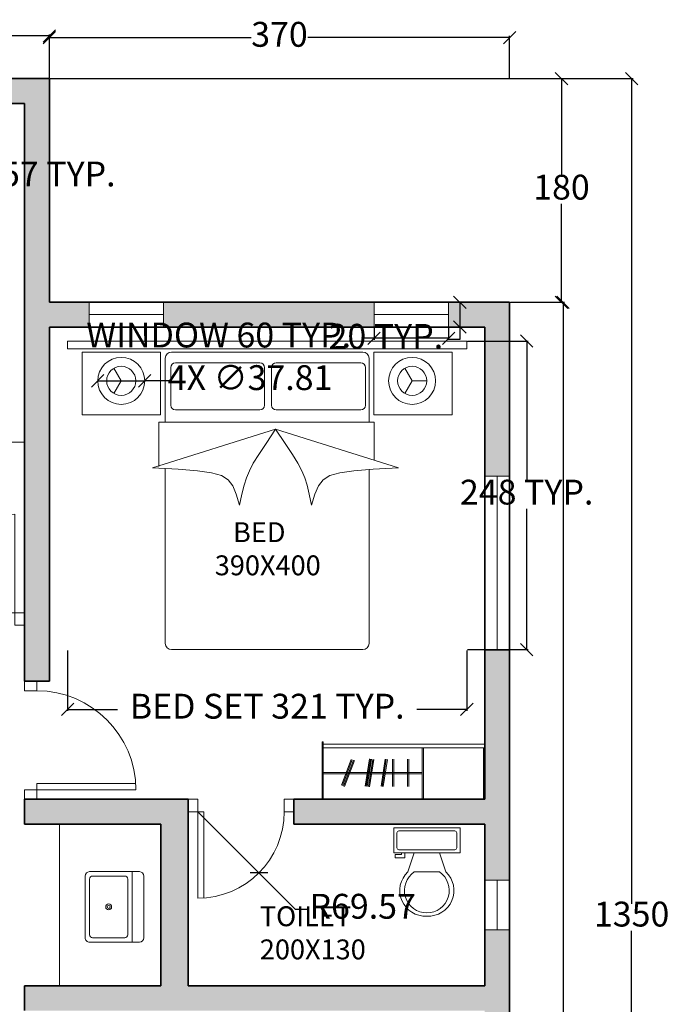
# Model space of a CAD drawing. Units: centimetres. Extents: x 2069 to 3209, y 376 to 1989.
# Tile 3 of 3: x 2687 to 3209, y 1196 to 1989. Entities that reach past the tile are written whole.
import ezdxf

# ---------------------------------------------------------------- set-up
doc = ezdxf.new("R2010")
doc.units = ezdxf.units.CM
for name, color, linetype, lineweight in [('A-ANNO-DIMS', 2, 'Continuous', 18), ('A-AREA-IDEN', 7, 'Continuous', 25), ('A-DOOR', 3, 'Continuous', 18), ('A-FLOR-CASE', 8, 'Continuous', 18), ('A-FLOR-FIXT', 8, 'Continuous', 18), ('A-FURN', 8, 'Continuous', 18), ('A-GLAZ', 4, 'Continuous', 18), ('A-WALL', 7, 'Continuous', 35), ('A-WALL-PATT', 252, 'Continuous', 13)]:
    doc.layers.add(name, color=color, linetype=linetype, lineweight=lineweight)
doc.styles.add('ATTR', font='romans.shx', dxfattribs={"width": 0.8, "height": 1.075})
doc.styles.get("Standard").update_dxf_attribs({"font": 'arial.ttf'})
doc.dimstyles.new('ISO-25', dxfattribs={"dimtxt": 20, "dimasz": 10, "dimexe": 1.25, "dimexo": 0.625, "dimtad": 0, "dimtih": 1, "dimtoh": 1, "dimtxsty": 'Standard', "dimblk": 'OBLIQUE', "dimcen": 6, "dimadec": 0, "dimazin": 0, "dimtfac": 1, "dimtmove": 0, "dimatfit": 3, "dimldrblk": 'OBLIQUE', "dimfxl": 1, "dimarcsym": 0})

# ---------------------------------------------------------------- blocks, each defined once
blk = doc.blocks.new('CAMMAT')
for p, q in [((1.2731, 0), (-1.2731, 0)), ((1.2731, 0), (1.2731, -0.05)), ((-1.2731, 0), (-1.2731, -0.05)), ((1.2731, -0.05), (-1.2731, -0.05)), ((-1.18, -0.07), (-1.18, -0.47)), ((-1.18, -0.07), (-0.68, -0.07)), ((-0.68, -0.07), (-0.68, -0.47)), ((-0.65, -0.11), (-0.65, -0.5169)), ((0.61, -0.07), (-0.61, -0.07)), ((0.65, -0.11), (0.65, -0.5169)), ((0.68, -0.07), (0.68, -0.47)), ((0.68, -0.07), (1.18, -0.07)), ((1.18, -0.07), (1.18, -0.47)), ((-0.931, -0.2541), (-0.9775, -0.1737)), ((-0.6152, -0.1695), (-0.6152, -0.4095)), ((-0.0465, -0.1395), (-0.5852, -0.1395)), ((-0.0165, -0.1695), (-0.0165, -0.4095)), ((0.0274, -0.1695), (0.0274, -0.4095)), ((0.5962, -0.1395), (0.0574, -0.1395)), ((0.6262, -0.1695), (0.6262, -0.4095)), ((0.9242, -0.2541), (0.8777, -0.1737)), ((-0.931, -0.2541), (-0.9775, -0.3346)), ((-0.931, -0.2541), (-0.8381, -0.2541)), ((0.9242, -0.2541), (0.8777, -0.3346)), ((0.9242, -0.2541), (1.0171, -0.2541)), ((-0.0465, -0.4395), (-0.5852, -0.4395)), ((0.5962, -0.4395), (0.0574, -0.4395)), ((-1.18, -0.47), (-0.68, -0.47)), ((0.68, -0.47), (1.18, -0.47)), ((0.0535, -0.5623), (-0.7312, -0.8093)), ((-0.6904, -0.5169), (-0.6904, -0.8)), ((-0.6904, -0.5169), (0.6826, -0.5169)), ((0.0535, -0.5623), (0.8382, -0.8093)), ((0.6826, -0.5169), (0.6826, -0.7603)), ((-0.65, -0.8139), (-0.65, -1.93)), ((0.65, -0.8204), (0.65, -1.93)), ((0.61, -1.97), (-0.61, -1.97))]:
    blk.add_line(p, q)
for points in [[(-0.1761, -1.0476), (-0.161, -0.9772), (-0.1474, -0.921), (-0.1326, -0.8732), (-0.1139, -0.8282), (-0.0886, -0.7803), (-0.0541, -0.7238), (-0.0076, -0.653), (0.0535, -0.5623)], [(0.2832, -1.0476), (0.2681, -0.9772), (0.2545, -0.921), (0.2396, -0.8732), (0.2209, -0.8282), (0.1957, -0.7803), (0.1611, -0.7238), (0.1147, -0.653), (0.0535, -0.5623)], [(-0.7312, -0.8093), (-0.5683, -0.8185), (-0.4451, -0.828), (-0.3552, -0.8406), (-0.2919, -0.8591), (-0.2489, -0.8862), (-0.2196, -0.9248), (-0.1975, -0.9777), (-0.1761, -1.0476)], [(0.8382, -0.8093), (0.6753, -0.8185), (0.5522, -0.828), (0.4622, -0.8406), (0.399, -0.8591), (0.356, -0.8862), (0.3267, -0.9248), (0.3046, -0.9777), (0.2832, -1.0476)]]:
    blk.add_lwpolyline(points)
for centre, radius in [((-0.931, -0.2541), 0.15), ((0.9242, -0.2541), 0.15), ((-0.931, -0.2541), 0.0929), ((0.9242, -0.2541), 0.0929)]:
    blk.add_circle(centre, radius)
for centre, radius, start, end in [((-0.61, -0.11), 0.04, 90, 180), ((0.61, -0.11), 0.04, 0, 90), ((-0.5852, -0.1695), 0.03, 90, 180), ((-0.0465, -0.1695), 0.03, 360, 90), ((0.0574, -0.1695), 0.03, 90, 180), ((0.5962, -0.1695), 0.03, 360, 90), ((-0.5852, -0.4095), 0.03, 180, 270), ((-0.0465, -0.4095), 0.03, 270, 360), ((0.0574, -0.4095), 0.03, 180, 270), ((0.5962, -0.4095), 0.03, 270, 360), ((-0.61, -1.93), 0.04, 180, 270), ((0.61, -1.93), 0.04, 270, 360)]:
    blk.add_arc(centre, radius, start, end)
blk = doc.blocks.new('*U10')
for p, q in [((241.3, -152.4), (241.3, -50.8)), ((-254, -215.9), (-203.2, -215.9)), ((-254, -241.3), (-254, -215.9)), ((-203.2, -215.9), (-203.2, -203.2)), ((-177.8, -203.2), (-177.8, -241.3)), ((-101.6, -203.2), (-152.4, -355.6)), ((101.6, -203.2), (152.4, -355.6)), ((-177.8, -241.3), (-254, -241.3)), ((101.6, -355.6), (-101.6, -355.6))]:
    blk.add_line(p, q)
blk.add_lwpolyline([(266.7, -203.2), (266.7, 0), (-266.7, 0), (-266.7, -203.2)], close=True)
for points in [[(-241.3, -50.8), (-241.3, -152.4)], [(215.9, -25.4), (-215.9, -25.4)], [(-215.9, -177.8), (215.9, -177.8)]]:
    blk.add_lwpolyline(points)
for centre, radius, start, end in [((-219.075, -47.625), 22.45064, 81.8699, 188.1301), ((219.075, -47.625), 22.45064, 351.8699, 98.1301), ((-219.075, -155.575), 22.45064, 171.869898, 278.1301), ((219.075, -155.575), 22.45064, 261.8699, 8.1301), ((-12.12088, -505.93752), 205.61935, 133.01722, 273.38), ((0.94996, -504.77674), 181.02486, 124.50543, 269.7), ((-0.94742, -504.77674), 181.02486, 270.3, 55.4946), ((12.12342, -505.93752), 205.61935, 266.62, 46.9828)]:
    blk.add_arc(centre, radius, start, end)
blk = doc.blocks.new("24'' Sink Single PV")
blk.add_line((-12.00001, -3.999996), (12, -3.999996))
for points in [[(-10.5, 0), (10.5, 0)], [(-12.00001, -18.499996), (-12.00001, -1.5)], [(12, -1.5), (12, -18.499996)], [(-10.5, -17.499996), (-10.5, -6.499996)], [(-9.5, -5.499996), (9.5, -5.499996)], [(10.5, -6.499996), (10.5, -17.499996)], [(10.5, -19.999996), (-10.5, -19.999996)], [(9.5, -18.499996), (-9.5, -18.499996)]]:
    blk.add_lwpolyline(points)
for radius in [1, 0.5]:
    blk.add_circle((0, -11.999996), radius)
for centre, radius, start, end in [((-10.5, -1.5), 1.5, 90, 180), ((10.5, -1.5), 1.5, 0, 90), ((-9.5, -6.499996), 1, 90, 180), ((9.5, -6.499996), 1, 0, 90), ((-10.5, -18.499996), 1.5, 180, 270), ((-9.5, -17.499996), 1, 180, 270), ((9.5, -17.499996), 1, 270, 0), ((10.5, -18.499996), 1.5, 270, 0)]:
    blk.add_arc(centre, radius, start, end)
at = {"style": 'ATTR', "width": 0.8, "flags": 9}
blk.add_attdef('ESTCODE', (0, 0), '', height=0.0048, dxfattribs=at)
blk = doc.blocks.new('_Oblique')
at = {"color": 0, "linetype": 'ByBlock', "lineweight": -2}
blk.add_line((-0.5, -0.5), (0.5, 0.5), dxfattribs=at)
blk = doc.blocks.new('*D11')
at = {"layer": 'A-ANNO-DIMS', "color": 0, "lineweight": -2, "transparency": 16777216}
for p, q in [((2320.39, 1941.81), (2320.39, 1976.68)), ((2320.39, 1975.43), (2492.71, 1975.43)), ((2710.39, 1975.43), (2538.06, 1975.43)), ((2710.39, 1941.81), (2710.39, 1976.68))]:
    blk.add_line(p, q, dxfattribs=at)
at = {"layer": 'Defpoints', "color": 0, "transparency": 16777216}
for p in [(2710.39, 1975.43), (2320.39, 1941.18), (2710.39, 1941.18)]:
    blk.add_point(p, dxfattribs=at)
at = {"layer": 'A-ANNO-DIMS', "color": 0, "lineweight": -2, "transparency": 16777216, "xscale": 10, "yscale": 10, "zscale": 10, "rotation": 180}
blk.add_blockref('_Oblique', (2320.39, 1975.43), dxfattribs=at)
at = {"layer": 'A-ANNO-DIMS', "color": 0, "lineweight": -2, "transparency": 16777216, "xscale": 10, "yscale": 10, "zscale": 10}
blk.add_blockref('_Oblique', (2710.39, 1975.43), dxfattribs=at)
at = {"layer": 'A-ANNO-DIMS', "color": 0, "transparency": 16777216, "insert": (2515.39, 1975.43), "char_height": 20, "attachment_point": 5}
blk.add_mtext('390', dxfattribs=at)
blk = doc.blocks.new('*D12')
at = {"layer": 'A-ANNO-DIMS', "color": 0, "lineweight": -2, "transparency": 16777216}
for p, q in [((2710.39, 1941.81), (2710.39, 1975.43)), ((2710.39, 1974.18), (2872.71, 1974.18)), ((3080.39, 1974.18), (2918.06, 1974.18)), ((3080.39, 1941.81), (3080.39, 1975.43))]:
    blk.add_line(p, q, dxfattribs=at)
at = {"layer": 'Defpoints', "color": 0, "transparency": 16777216}
for p in [(3080.39, 1974.18), (2710.39, 1941.18), (3080.39, 1941.18)]:
    blk.add_point(p, dxfattribs=at)
at = {"layer": 'A-ANNO-DIMS', "color": 0, "lineweight": -2, "transparency": 16777216, "xscale": 10, "yscale": 10, "zscale": 10, "rotation": 180}
blk.add_blockref('_Oblique', (2710.39, 1974.18), dxfattribs=at)
at = {"layer": 'A-ANNO-DIMS', "color": 0, "lineweight": -2, "transparency": 16777216, "xscale": 10, "yscale": 10, "zscale": 10}
blk.add_blockref('_Oblique', (3080.39, 1974.18), dxfattribs=at)
at = {"layer": 'A-ANNO-DIMS', "color": 0, "transparency": 16777216, "insert": (2895.39, 1974.18), "char_height": 20, "attachment_point": 5}
blk.add_mtext('370', dxfattribs=at)
blk = doc.blocks.new('*D15')
at = {"layer": 'A-ANNO-DIMS', "color": 0, "lineweight": -2, "transparency": 16777216}
for p, q in [((3081.01, 1941.18), (3123.32, 1941.18)), ((3122.07, 1941.18), (3122.07, 1862.02)), ((3122.07, 1761.18), (3122.07, 1840.35)), ((3081.01, 1761.18), (3123.32, 1761.18))]:
    blk.add_line(p, q, dxfattribs=at)
at = {"layer": 'Defpoints', "color": 0, "transparency": 16777216}
for p in [(3080.39, 1941.18), (3080.39, 1761.18), (3122.07, 1761.18)]:
    blk.add_point(p, dxfattribs=at)
at = {"layer": 'A-ANNO-DIMS', "color": 0, "lineweight": -2, "transparency": 16777216, "xscale": 10, "yscale": 10, "zscale": 10}
for p, rotation in [((3122.07, 1941.18), 90), ((3122.07, 1761.18), 270)]:
    blk.add_blockref('_Oblique', p, dxfattribs=dict(at, rotation=rotation))
at = {"layer": 'A-ANNO-DIMS', "color": 0, "transparency": 16777216, "insert": (3122.07, 1851.18), "char_height": 20, "attachment_point": 5}
blk.add_mtext('180', dxfattribs=at)
blk = doc.blocks.new('*D16')
at = {"layer": 'A-ANNO-DIMS', "color": 0, "lineweight": -2, "transparency": 16777216}
for p, q in [((3081.01, 1761.18), (3124.57, 1761.18)), ((3123.32, 1761.18), (3123.32, 1187.02)), ((3123.32, 591.18), (3123.32, 1165.35)), ((3081.01, 591.18), (3124.57, 591.18))]:
    blk.add_line(p, q, dxfattribs=at)
at = {"layer": 'Defpoints', "color": 0, "transparency": 16777216}
for p in [(3080.39, 1761.18), (3080.39, 591.18), (3123.32, 591.18)]:
    blk.add_point(p, dxfattribs=at)
at = {"layer": 'A-ANNO-DIMS', "color": 0, "lineweight": -2, "transparency": 16777216, "xscale": 10, "yscale": 10, "zscale": 10}
for p, rotation in [((3123.32, 1761.18), 90), ((3123.32, 591.18), 270)]:
    blk.add_blockref('_Oblique', p, dxfattribs=dict(at, rotation=rotation))
at = {"layer": 'A-ANNO-DIMS', "color": 0, "transparency": 16777216, "insert": (3123.32, 1176.18), "char_height": 20, "attachment_point": 5}
blk.add_mtext('1170', dxfattribs=at)
blk = doc.blocks.new('WIN-600')
for p, q in [((0, 20), (0, 0)), ((60, 20), (60, 0)), ((60, 10), (0, 10))]:
    blk.add_line(p, q)
blk = doc.blocks.new('WIN-1400')
for p, q in [((0, 140), (20, 140)), ((10, 0), (10, 140)), ((0, 0), (20, 0))]:
    blk.add_line(p, q)
blk = doc.blocks.new('DOOR-SINGLE-950')
for p, q in [((82.28, 89.41), (82.28, 10)), ((87.28, 89.57), (87.28, 10)), ((0, 10), (7.71, 10)), ((7.71, 10), (7.71, 0)), ((82.28, 10), (87.28, 10)), ((95, 10), (87.28, 10)), ((87.28, 10), (87.28, 0)), ((7.71, 0), (0, 0)), ((87.28, 0), (95, 0))]:
    blk.add_line(p, q)
blk.add_arc((87.28, 10), 79.57, 90, 180)
blk = doc.blocks.new('*D36')
at = {"layer": 'A-ANNO-DIMS', "color": 0, "lineweight": -2, "transparency": 16777216}
for p, q in [((2531.27, 1869.68), (2531.27, 1860.55)), ((2587.96, 1869.68), (2587.96, 1860.55)), ((2531.27, 1861.8), (2587.96, 1861.8)), ((2587.96, 1861.8), (2597.96, 1861.8))]:
    blk.add_line(p, q, dxfattribs=at)
at = {"layer": 'Defpoints', "color": 0, "transparency": 16777216}
for p in [(2531.27, 1870.31), (2587.96, 1870.31), (2587.96, 1861.8)]:
    blk.add_point(p, dxfattribs=at)
at = {"layer": 'A-ANNO-DIMS', "color": 0, "lineweight": -2, "transparency": 16777216, "xscale": 10, "yscale": 10, "zscale": 10, "rotation": 180}
blk.add_blockref('_Oblique', (2531.27, 1861.8), dxfattribs=at)
at = {"layer": 'A-ANNO-DIMS', "color": 0, "lineweight": -2, "transparency": 16777216, "xscale": 10, "yscale": 10, "zscale": 10}
blk.add_blockref('_Oblique', (2587.96, 1861.8), dxfattribs=at)
at = {"layer": 'A-ANNO-DIMS', "color": 0, "transparency": 16777216, "insert": (2683.7, 1861.8), "char_height": 20, "attachment_point": 5}
blk.add_mtext('SINK 57 TYP.', dxfattribs=at)
blk = doc.blocks.new('*D40')
at = {"layer": 'A-ANNO-DIMS', "color": 0, "lineweight": -2, "transparency": 16777216}
for p, q in [((2725.06, 1481.01), (2725.06, 1432.25)), ((3045.99, 1481.01), (3045.99, 1432.25)), ((2725.06, 1433.5), (2765.24, 1433.5)), ((3045.99, 1433.5), (3005.81, 1433.5))]:
    blk.add_line(p, q, dxfattribs=at)
at = {"layer": 'Defpoints', "color": 0, "transparency": 16777216}
for p in [(2725.06, 1481.63), (3045.99, 1481.63), (3045.99, 1433.5)]:
    blk.add_point(p, dxfattribs=at)
at = {"layer": 'A-ANNO-DIMS', "color": 0, "lineweight": -2, "transparency": 16777216, "xscale": 10, "yscale": 10, "zscale": 10, "rotation": 180}
blk.add_blockref('_Oblique', (2725.06, 1433.5), dxfattribs=at)
at = {"layer": 'A-ANNO-DIMS', "color": 0, "lineweight": -2, "transparency": 16777216, "xscale": 10, "yscale": 10, "zscale": 10}
blk.add_blockref('_Oblique', (3045.99, 1433.5), dxfattribs=at)
at = {"layer": 'A-ANNO-DIMS', "color": 0, "transparency": 16777216, "insert": (2885.52, 1433.5), "char_height": 20, "attachment_point": 5}
blk.add_mtext('BED SET 321 TYP.', dxfattribs=at)
blk = doc.blocks.new('*D41')
at = {"layer": 'A-ANNO-DIMS', "color": 0, "lineweight": -2, "transparency": 16777216}
for p, q in [((3046.61, 1729.93), (3095.37, 1729.93)), ((3094.12, 1729.93), (3094.12, 1616.62)), ((3094.12, 1481.63), (3094.12, 1594.94)), ((3046.61, 1481.63), (3095.37, 1481.63))]:
    blk.add_line(p, q, dxfattribs=at)
at = {"layer": 'Defpoints', "color": 0, "transparency": 16777216}
for p in [(3045.99, 1729.93), (3094.12, 1729.93), (3045.99, 1481.63)]:
    blk.add_point(p, dxfattribs=at)
at = {"layer": 'A-ANNO-DIMS', "color": 0, "lineweight": -2, "transparency": 16777216, "xscale": 10, "yscale": 10, "zscale": 10}
for p, rotation in [((3094.12, 1729.93), 90), ((3094.12, 1481.63), 270)]:
    blk.add_blockref('_Oblique', p, dxfattribs=dict(at, rotation=rotation))
at = {"layer": 'A-ANNO-DIMS', "color": 0, "transparency": 16777216, "insert": (3094.12, 1605.78), "char_height": 20, "attachment_point": 5}
blk.add_mtext('248 TYP.', dxfattribs=at)
blk = doc.blocks.new('*D42')
at = {"layer": 'A-ANNO-DIMS', "color": 0, "lineweight": -2, "transparency": 16777216}
for p, q in [((2971.39, 1740.56), (2971.39, 1730.93)), ((3031.39, 1740.56), (3031.39, 1730.93)), ((2971.39, 1732.18), (2961.39, 1732.18)), ((3031.39, 1732.18), (2971.39, 1732.18))]:
    blk.add_line(p, q, dxfattribs=at)
at = {"layer": 'Defpoints', "color": 0, "transparency": 16777216}
for p in [(2971.39, 1741.18), (3031.39, 1741.18), (2971.39, 1732.18)]:
    blk.add_point(p, dxfattribs=at)
at = {"layer": 'A-ANNO-DIMS', "color": 0, "lineweight": -2, "transparency": 16777216, "xscale": 10, "yscale": 10, "zscale": 10, "rotation": 180}
blk.add_blockref('_Oblique', (2971.39, 1732.18), dxfattribs=at)
at = {"layer": 'A-ANNO-DIMS', "color": 0, "lineweight": -2, "transparency": 16777216, "xscale": 10, "yscale": 10, "zscale": 10}
blk.add_blockref('_Oblique', (3031.39, 1732.18), dxfattribs=at)
at = {"layer": 'A-ANNO-DIMS', "color": 0, "transparency": 16777216, "insert": (2846.5, 1732.18), "char_height": 20, "attachment_point": 5}
blk.add_mtext('WINDOW 60 TYP.', dxfattribs=at)
blk = doc.blocks.new('*D43')
at = {"layer": 'A-ANNO-DIMS', "color": 0, "lineweight": -2, "transparency": 16777216}
for p, q in [((3032.01, 1761.18), (3041.64, 1761.18)), ((3040.39, 1761.18), (3040.39, 1741.18)), ((3032.01, 1741.18), (3041.64, 1741.18)), ((3040.39, 1741.18), (3040.39, 1731.18)), ((3040.39, 1731.18), (3030.39, 1731.18))]:
    blk.add_line(p, q, dxfattribs=at)
at = {"layer": 'Defpoints', "color": 0, "transparency": 16777216}
for p in [(3031.39, 1761.18), (3031.39, 1741.18), (3040.39, 1741.18)]:
    blk.add_point(p, dxfattribs=at)
at = {"layer": 'A-ANNO-DIMS', "color": 0, "lineweight": -2, "transparency": 16777216, "xscale": 10, "yscale": 10, "zscale": 10}
for p, rotation in [((3040.39, 1761.18), 90), ((3040.39, 1741.18), 270)]:
    blk.add_blockref('_Oblique', p, dxfattribs=dict(at, rotation=rotation))
at = {"layer": 'A-ANNO-DIMS', "color": 0, "transparency": 16777216, "insert": (2980.92, 1731.18), "char_height": 20, "attachment_point": 5}
blk.add_mtext('20 TYP.', dxfattribs=at)
blk = doc.blocks.new('*D47')
at = {"layer": 'A-ANNO-DIMS', "color": 0, "lineweight": -2, "transparency": 16777216}
for p, q in [((2711.01, 1941.18), (3179.73, 1941.18)), ((3178.48, 1941.18), (3178.48, 1277.03)), ((3178.48, 591.18), (3178.48, 1255.34)), ((3081.01, 591.18), (3179.73, 591.18))]:
    blk.add_line(p, q, dxfattribs=at)
at = {"layer": 'Defpoints', "color": 0, "transparency": 16777216}
for p in [(2710.39, 1941.18), (3080.39, 591.18), (3178.48, 591.18)]:
    blk.add_point(p, dxfattribs=at)
at = {"layer": 'A-ANNO-DIMS', "color": 0, "lineweight": -2, "transparency": 16777216, "xscale": 10, "yscale": 10, "zscale": 10}
for p, rotation in [((3178.48, 1941.18), 90), ((3178.48, 591.18), 270)]:
    blk.add_blockref('_Oblique', p, dxfattribs=dict(at, rotation=rotation))
at = {"layer": 'A-ANNO-DIMS', "color": 0, "transparency": 16777216, "insert": (3178.48, 1266.18), "char_height": 20, "attachment_point": 5}
blk.add_mtext('1350', dxfattribs=at)
blk = doc.blocks.new('*D51')
at = {"layer": 'A-ANNO-DIMS', "color": 0, "lineweight": -2, "transparency": 16777216}
for p, q in [((2829.62, 1351.18), (2878.82, 1301.99)), ((2908.33, 1272.47), (2878.82, 1301.99)), ((2918.33, 1272.47), (2908.33, 1272.47))]:
    blk.add_line(p, q, dxfattribs=at)
at = {"layer": 'Defpoints', "color": 0, "transparency": 16777216}
for p in [(2829.62, 1351.18), (2878.82, 1301.99)]:
    blk.add_point(p, dxfattribs=at)
at = {"layer": 'A-ANNO-DIMS', "color": 0, "lineweight": -2, "transparency": 16777216, "xscale": 10, "yscale": 10, "zscale": 10, "rotation": 135.0001607294283}
blk.add_blockref('_Oblique', (2878.82, 1301.99), dxfattribs=at)
at = {"layer": 'A-ANNO-DIMS', "color": 0, "transparency": 16777216, "insert": (2962.27, 1272.47), "char_height": 20, "attachment_point": 5}
blk.add_mtext('R69.57', dxfattribs=at)
blk = doc.blocks.new('*D52')
at = {"layer": 'A-ANNO-DIMS', "color": 0, "lineweight": -2, "transparency": 16777216}
for p in [(2749.27, 1697.9), (2807.08, 1697.9)]:
    blk.add_line(p, (2787.08, 1697.9), dxfattribs=at)
at = {"layer": 'Defpoints', "color": 0, "transparency": 16777216}
for p in [(2749.27, 1697.9), (2787.08, 1697.9)]:
    blk.add_point(p, dxfattribs=at)
at = {"layer": 'A-ANNO-DIMS', "color": 0, "lineweight": -2, "transparency": 16777216, "xscale": 10, "yscale": 10, "zscale": 10}
for p, rotation in [((2749.27, 1697.9), 0.0014516758650363), ((2787.08, 1697.9), 180.001451675865)]:
    blk.add_blockref('_Oblique', p, dxfattribs=dict(at, rotation=rotation))
at = {"layer": 'A-ANNO-DIMS', "color": 0, "transparency": 16777216, "insert": (2871.76, 1697.9), "char_height": 20, "attachment_point": 5}
blk.add_mtext('4X ∅37.81', dxfattribs=at)

msp = doc.modelspace()

# ---------------------------------------------------------------- hatches: boundary and pattern name
at = {"layer": 'A-WALL-PATT'}
h = msp.add_hatch(color=256, dxfattribs=at)
h.dxf.hatch_style = 1
h.paths.add_polyline_path([(2498.1872, 1921.1819), (2498.1872, 1941.1819), (2320.3865, 1941.1819), (2320.3865, 1616.1819), (2340.3865, 1616.1819), (2340.3865, 1921.1819)])
h.paths.add_polyline_path([(2690.3865, 1921.1819), (2690.3865, 1456.1819), (2710.3865, 1456.1819), (2710.3865, 1741.1819), (2742.2674, 1741.1819), (2742.2674, 1761.1819), (2710.3865, 1761.1819), (2710.3865, 1941.1819), (2618.1872, 1941.1819), (2618.1872, 1921.1819)])
h.paths.add_polyline_path([(2802.2674, 1761.1819), (2802.2674, 1741.1819), (2971.3879, 1741.1819), (2971.3879, 1761.1819)])
h.paths.add_polyline_path([(3080.3865, 1761.1819), (3031.3879, 1761.1819), (3031.3879, 1741.1819), (3060.3865, 1741.1819), (3060.3865, 1621.1819), (3080.3865, 1621.1819)])
h.paths.add_polyline_path([(3060.3865, 1361.1819), (2906.9077, 1361.1819), (2906.9077, 1341.1819), (3060.3865, 1341.1819), (3060.3865, 1296.1819), (3080.3865, 1296.1819), (3080.3865, 1481.1819), (3060.3865, 1481.1819)])
h.paths.add_polyline_path([(2799.9077, 1341.1819), (2799.9077, 1211.1819), (2690.3865, 1211.1819), (2690.3865, 1191.1819), (3060.3865, 1191.1819), (3060.3865, 1131.1819), (3080.3865, 1131.1819), (3080.3865, 1256.1819), (3060.3865, 1256.1819), (3060.3865, 1211.1819), (2821.9077, 1211.1819), (2821.9077, 1361.1819), (2690.3865, 1361.1819), (2690.3865, 1341.1819)])
h.paths.add_polyline_path([(3080.3865, 1051.1819), (3060.3865, 1051.1819), (3060.3865, 991.1819), (2805.3865, 991.1819), (2805.3865, 971.1819), (3060.3865, 971.1819), (3060.3865, 861.1819), (3080.3865, 861.1819)])
h.paths.add_polyline_path([(2690.3865, 591.1819), (2815.3865, 591.1819), (2815.3865, 611.1819), (2710.3865, 611.1819), (2710.3865, 991.1819), (2690.3865, 991.1819)])
h.paths.add_polyline_path([(2955.3865, 611.1819), (2955.3865, 591.1819), (3080.3865, 591.1819), (3080.3865, 721.1819), (3060.3865, 721.1819), (3060.3865, 611.1819)])
h.paths.add_polyline_path([(2320.3865, 656.2562), (2320.3865, 639.1819), (2343.1963, 639.1819), (2343.1963, 656.2562)])
h.paths.add_polyline_path([(2320.3865, 863.2574), (2250.3865, 863.2574), (2250.3865, 841.2574), (2407.8865, 841.2574), (2407.8865, 863.2574), (2340.3865, 863.2574), (2340.3865, 927.2197), (2320.3865, 927.2197)])
h.paths.add_polyline_path([(2320.3865, 1151.1819), (2320.3865, 1087.2197), (2340.3865, 1087.2197), (2340.3865, 1151.1819), (2595.3865, 1151.1819), (2595.3865, 1171.1819), (2270.3865, 1171.1819), (2270.3865, 1216.1819), (2180.3865, 1216.1819), (2180.3865, 1196.1819), (2250.3865, 1196.1819), (2250.3865, 1151.1819)])
h.paths.add_polyline_path([(2595.3865, 1501.1819), (2595.3865, 1521.1819), (2250.3865, 1521.1819), (2250.3865, 1476.1819), (2180.3865, 1476.1819), (2180.3865, 1456.1819), (2270.3865, 1456.1819), (2270.3865, 1501.1819)])

# ---------------------------------------------------------------- linework, layer by layer
at = {"layer": 'A-DOOR'}
for p, q in [((2821.9077, 1361.1819), (2829.6228, 1361.1819)), ((2829.6228, 1361.1819), (2829.6228, 1351.1819)), ((2906.9077, 1361.1819), (2899.1927, 1361.1819)), ((2899.1927, 1361.1819), (2899.1927, 1351.1819)), ((2829.6228, 1351.1819), (2821.9077, 1351.1819)), ((2829.6228, 1351.1819), (2829.6228, 1281.612)), ((2834.6228, 1351.1819), (2829.6228, 1351.1819)), ((2834.6228, 1351.1819), (2834.6228, 1281.7919)), ((2899.1927, 1351.1819), (2906.9077, 1351.1819))]:
    msp.add_line(p, q, dxfattribs=at)
msp.add_arc((2829.6228, 1351.1819), 69.5699, 270, 0, dxfattribs=at)
at = {"layer": 'A-FLOR-CASE'}
for p, q in [((2630.3865, 1648.6184), (2690.3865, 1648.6184)), ((2929.621, 1361.1819), (2929.621, 1407.5284)), ((2929.621, 1407.5284), (2930.621, 1407.5284)), ((2930.621, 1407.5284), (2930.621, 1405.5284)), ((2930.621, 1405.5284), (3060.3865, 1405.5284)), ((2930.621, 1405.5284), (2930.621, 1405.5284)), ((2930.621, 1405.5284), (2930.621, 1361.1819)), ((2930.621, 1402.5284), (3060.3865, 1402.5284)), ((3010.122, 1361.1819), (3010.122, 1402.5284)), ((3011.122, 1361.1819), (3011.122, 1402.5284)), ((3059.3865, 1361.1819), (3059.3865, 1402.5284)), ((3060.3865, 1361.1819), (3060.3865, 1405.5284)), ((2945.2037, 1372.503), (2953.0892, 1393.2295)), ((2946.0458, 1372.1827), (2953.9313, 1392.9091)), ((2946.8878, 1371.8623), (2954.7733, 1392.5888)), ((2947.7299, 1371.5419), (2955.6154, 1392.2684)), ((2964.1632, 1371.7675), (2967.6894, 1393.6612)), ((2965.0527, 1371.6242), (2968.5789, 1393.5179)), ((2965.9422, 1371.4809), (2969.4684, 1393.3747)), ((2966.8317, 1371.3377), (2970.3578, 1393.2314)), ((2967.7212, 1371.1944), (2971.2473, 1393.0881)), ((2977.0375, 1371.6042), (2980.3959, 1393.5243)), ((2977.928, 1371.4678), (2981.2865, 1393.3878)), ((2978.8186, 1371.3313), (2982.177, 1393.2514)), ((2986.3288, 1371.3399), (2986.3288, 1393.5157)), ((2987.2297, 1371.3399), (2987.2297, 1393.5157)), ((2998.3848, 1371.3399), (2998.3848, 1393.5157)), ((2999.2858, 1371.3399), (2999.2858, 1393.5157)), ((2930.621, 1382.7423), (3010.122, 1382.7423)), ((2930.621, 1381.7423), (3010.122, 1381.7423)), ((2718.6731, 1341.1819), (2718.6731, 1211.1819))]:
    msp.add_line(p, q, dxfattribs=at)
at = {"layer": 'A-GLAZ'}
for p, q in [((3060.3865, 1296.1819), (3080.3865, 1296.1819)), ((3070.3865, 1256.1819), (3070.3865, 1296.1819)), ((3060.3865, 1256.1819), (3080.3865, 1256.1819))]:
    msp.add_line(p, q, dxfattribs=at)
at = {"layer": 'A-WALL'}
for p, q in [((2320.3865, 1941.1819), (2710.3865, 1941.1819)), ((2710.3865, 1941.1819), (2710.3865, 1761.1819)), ((2340.3865, 1921.1819), (2690.3865, 1921.1819)), ((2690.3865, 1921.1819), (2690.3865, 1456.1819)), ((2710.3865, 1761.1819), (3080.3865, 1761.1819)), ((3080.3865, 1761.1819), (3080.3865, 591.1819)), ((2710.3865, 1741.1819), (3060.3865, 1741.1819)), ((2710.3865, 1741.1819), (2710.3865, 1456.1819)), ((3060.3865, 1741.1819), (3060.3865, 1361.1819)), ((2690.3865, 1456.1819), (2710.3865, 1456.1819)), ((2690.3865, 1361.1819), (2821.9077, 1361.1819)), ((2690.3865, 1361.1819), (2690.3865, 1341.1819)), ((2821.9077, 1361.1819), (2821.9077, 1211.1819)), ((2906.9077, 1361.1819), (2906.9077, 1341.1819)), ((2906.9077, 1361.1819), (3060.3865, 1361.1819)), ((2690.3865, 1341.1819), (2799.9077, 1341.1819)), ((2799.9077, 1341.1819), (2799.9077, 1211.1819)), ((2906.9077, 1341.1819), (3060.3865, 1341.1819)), ((3060.3865, 1341.1819), (3060.3865, 1211.1819)), ((2690.3865, 1211.1819), (2799.9077, 1211.1819)), ((2690.3865, 1211.1819), (2690.3865, 1191.1819)), ((2821.9077, 1211.1819), (3060.3865, 1211.1819))]:
    msp.add_line(p, q, dxfattribs=at)

# ---------------------------------------------------------------- block references
at = {"layer": 'A-DOOR'}
msp.add_blockref('DOOR-SINGLE-950', (2595.387, 1501.182), dxfattribs=at)
at = {"layer": 'A-DOOR', "rotation": 269.9999999999998}
msp.add_blockref('DOOR-SINGLE-950', (2690.3866, 1456.1815), dxfattribs=at)
at = {"layer": 'A-FLOR-FIXT', "xscale": 0.1, "yscale": 0.1, "zscale": 0.1}
msp.add_blockref('*U10', (3013.8552, 1338.3054), dxfattribs=at)
at = {"layer": 'A-FLOR-FIXT', "xscale": 2.362111345995379, "yscale": 2.362111345995379, "zscale": 2.362111345995379, "rotation": 270}
msp.add_blockref("24'' Sink Single PV", (2786.4165, 1274.5809), dxfattribs=at)
at = {"layer": 'A-FURN', "xscale": 126.0367650401743, "yscale": 126.0367650401743, "zscale": 126.0367650401743}
msp.add_blockref('CAMMAT', (2885.5243, 1729.9268), dxfattribs=at)
at = {"layer": 'A-GLAZ'}
for name, p in [('WIN-600', (2742.2675, 1741.182)), ('WIN-1400', (3060.387, 1481.182))]:
    msp.add_blockref(name, p, dxfattribs=at)
at = {"layer": 'A-GLAZ', "rotation": 180}
msp.add_blockref('WIN-600', (3031.3878, 1761.1818), dxfattribs=at)

# ---------------------------------------------------------------- texts
at = {"layer": 'A-AREA-IDEN', "char_height": 16, "attachment_point": 1}
for s, width, insert in [('   BED\\P390X400', 126.109071, (2843.3575, 1584.1102)), ('TOILET\\P200X130', 83.87785, (2879.5688, 1275.0364))]:
    msp.add_mtext_dynamic_manual_height_columns(s, width=width, gutter_width=12.5, heights=[0], dxfattribs=dict(at, insert=insert))

# ---------------------------------------------------------------- dimensions: what is measured, and where the dimension line sits
at = {"layer": 'A-ANNO-DIMS'}
for base, p1, p2, picture, middle in [((2710.3865, 1975.4288), (2320.3865, 1941.1819), (2710.3865, 1941.1819), '*D11', (2515.3865, 1975.4288)), ((3080.3865, 1974.1788), (2710.3865, 1941.1819), (3080.3865, 1941.1819), '*D12', (2895.3865, 1974.1788))]:
    dim = msp.add_linear_dim(base=base, p1=p1, p2=p2, dimstyle='ISO-25', override={"dimclrd": 0, "dimclre": 0, "dimclrt": 0}, dxfattribs=at)
    dim.commit()
    dim.dimension.update_dxf_attribs({"geometry": picture, "text_midpoint": middle})
for base, p1, p2, override, picture, middle in [((3178.4752, 591.1819), (2710.3865, 1941.1819), (3080.3865, 591.1819), {"dimdec": 0, "dimlfac": 1, "dimrnd": 0, "dimzin": 0, "dimdsep": 46, "dimlunit": 2}, '*D47', (3178.4752, 1266.1819)), ((3122.0686, 1761.1819), (3080.3865, 1941.1819), (3080.3865, 1761.1819), {"dimclrd": 0, "dimclre": 0, "dimclrt": 0}, '*D15', (3122.0686, 1851.1819)), ((3123.3186, 591.1819), (3080.3865, 1761.1819), (3080.3865, 591.1819), {"dimclrd": 0, "dimclre": 0, "dimclrt": 0}, '*D16', (3123.3186, 1176.1819))]:
    dim = msp.add_linear_dim(base=base, p1=p1, p2=p2, angle=90, dimstyle='ISO-25', override=override, dxfattribs=at)
    dim.commit()
    dim.dimension.update_dxf_attribs({"geometry": picture, "text_midpoint": middle})
for base, p1, p2, text, picture, middle in [((2587.9624, 1861.8033), (2531.2717, 1870.3069), (2587.9624, 1870.3069), 'SINK <> TYP.', '*D36', (2683.7034, 1861.8033)), ((3045.9858, 1433.4959), (2725.0627, 1481.6344), (3045.9858, 1481.6344), 'BED SET <> TYP.', '*D40', (2885.5243, 1433.4959))]:
    dim = msp.add_linear_dim(base=base, p1=p1, p2=p2, text=text, dimstyle='ISO-25', override={"dimdec": 0, "dimlfac": 1, "dimrnd": 0, "dimzin": 0, "dimdsep": 46, "dimlunit": 2}, dxfattribs=at)
    dim.commit()
    dim.dimension.update_dxf_attribs({"geometry": picture, "text_midpoint": middle})
for base, p1, p2, angle, text, picture, middle in [((2971.3879, 1732.1819), (3031.3879, 1741.1819), (2971.3879, 1741.1819), 180, 'WINDOW <> TYP.', '*D42', (2846.4996, 1732.1819)), ((3040.3879, 1741.1819), (3031.3879, 1761.1819), (3031.3879, 1741.1819), 270, '<> TYP.', '*D43', (2980.9157, 1731.1819)), ((3094.1243, 1729.9268), (3045.9858, 1481.6344), (3045.9858, 1729.9268), 90, '<> TYP.', '*D41', (3094.1243, 1605.7806))]:
    dim = msp.add_linear_dim(base=base, p1=p1, p2=p2, angle=angle, text=text, dimstyle='ISO-25', override={"dimdec": 0, "dimlfac": 1, "dimrnd": 0, "dimzin": 0, "dimdsep": 46, "dimlunit": 2}, dxfattribs=at)
    dim.commit()
    dim.dimension.update_dxf_attribs({"geometry": picture, "text_midpoint": middle})
dim = msp.add_diameter_dim_2p(p1=(2749.2737, 1697.9), p2=(2787.0847, 1697.901), text='4X <>', dimstyle='ISO-25', override={"dimdec": 2, "dimlfac": 1, "dimrnd": 0, "dimzin": 0, "dimdsep": 46, "dimlunit": 2}, dxfattribs=at)
dim.commit()
dim.dimension.update_dxf_attribs({"geometry": '*D52', "text_midpoint": (2807.0847, 1697.9015), "dimtype": 163})
dim = msp.add_radius_dim(center=(2829.6228, 1351.1819), mpoint=(2878.8163, 1301.9887), dimstyle='ISO-25', override={"dimdec": 2, "dimlfac": 1, "dimrnd": 0, "dimzin": 0, "dimdsep": 46, "dimlunit": 2}, dxfattribs=at)
dim.commit()
dim.dimension.update_dxf_attribs({"geometry": '*D51', "text_midpoint": (2962.2725, 1272.4728), "dimtype": 164})

doc.saveas('drawing.dxf')
